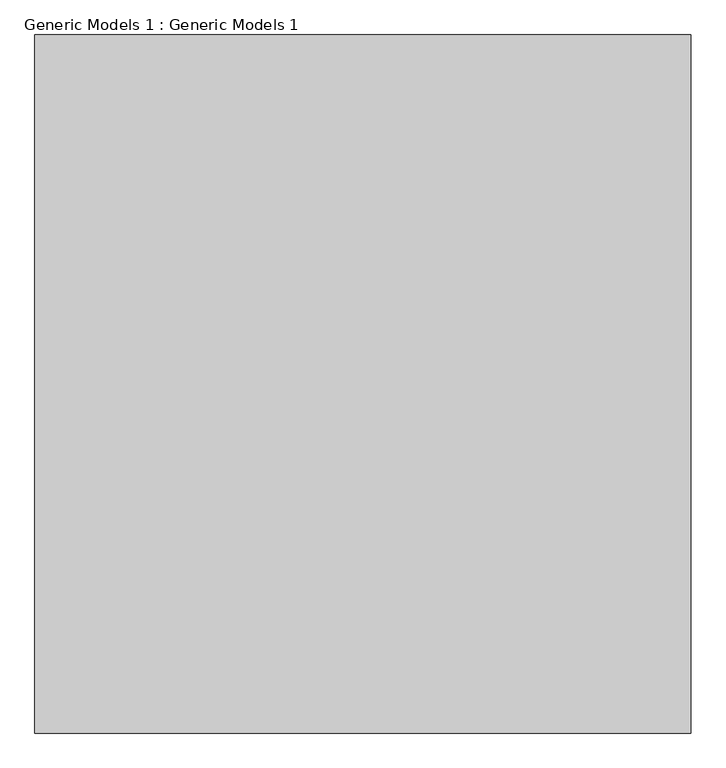
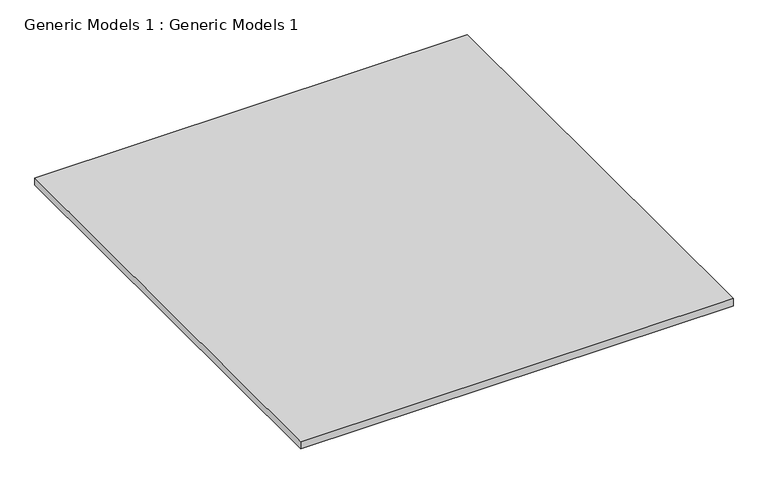
"""IFC4 building model written with IfcOpenShell, lengths in millimetres: proxy geometry, Generic Models 1 : Generic Models 1."""

from ifc_helpers import new_model, si_unit, frame, origin, place, context, project, spatial, polyline, outline, extrude, source, transform, mapped, element, save


def generic_models_1_generic_models_1_28fb3979(model_context):
    return source(origin(), model_context, "Body", "SweptSolid", [
        extrude(outline(polyline([(-4576.7695233, 1742.5041488), (-4576.7695233, -16496.9752569), (-21722.1696364, -16496.9752569), (-21722.1696364, 1742.5041488), (-4576.7695233, 1742.5041488)])), frame((0.0, 0.0, -304.8), z_axis=(0.0, 0.0, 1.0), x_axis=(1.0, 0.0, 0.0)), (0.0, 0.0, 1.0), 304.8),
    ])


if __name__ == "__main__":
    model = new_model("IFC4")
    model_context = context("Model", 3, world=origin())
    ifc_project = project(units=[si_unit("LENGTHUNIT", "METRE", prefix="MILLI")], contexts=[model_context])
    site = spatial("IfcSite", under=ifc_project)
    building = spatial("IfcBuilding", under=site)
    placement = place(None, origin())
    generic_models_1_generic_models_1_shape = generic_models_1_generic_models_1_28fb3979(model_context)
    element("IfcBuildingElementProxy", 1, Name="Generic Models 1 : Generic Models 1", ObjectType="Generic Models 1 : Generic Models 1", at=placement, inside=building, context=model_context, shape_type="MappedRepresentation", body=[
        mapped(generic_models_1_generic_models_1_shape, transform((0.0, 0.0, 0.0), x_axis=(1.0, 0.0, 0.0), y_axis=(0.0, 1.0, 0.0), z_axis=(0.0, 0.0, 1.0))),
    ])
    save(model, "model.ifc")
